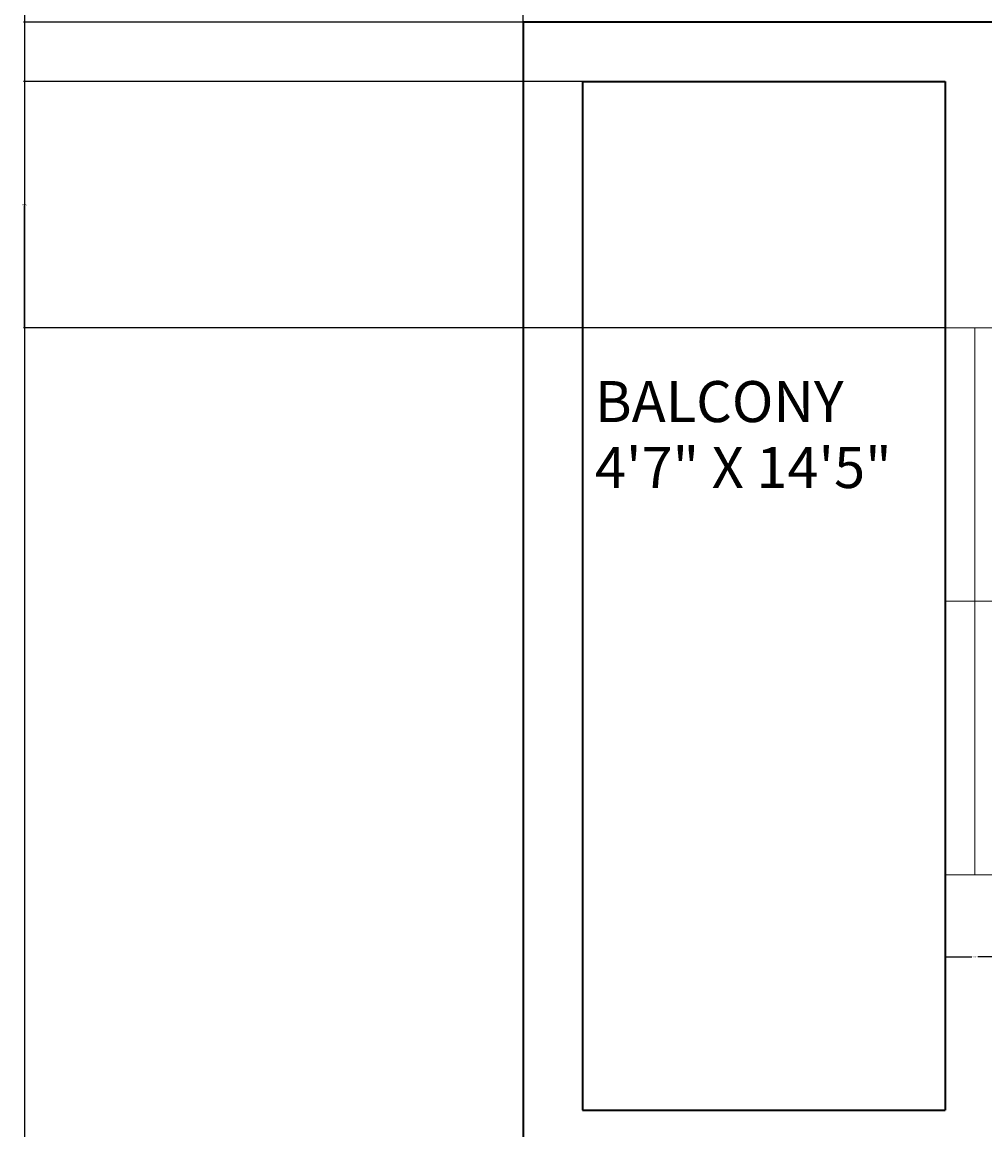
# Model space of a CAD drawing. Units: inches. Extents: x -61 to 1599, y -1316 to 257.
# Tile 112 of 204: x -61 to 85, y -10 to 158. Entities that reach past the tile are written whole.
import ezdxf

# ---------------------------------------------------------------- set-up
doc = ezdxf.new("R2010")
doc.units = ezdxf.units.IN
doc.header["$MEASUREMENT"] = 0
for name, color, linetype, lineweight in [('A-ANNO-DIMS', 2, 'Continuous', 18), ('A-AREA-IDEN', 1, 'Continuous', 18), ('WALLS', 4, 'Continuous', 35), ('WINDOWS', 220, 'Continuous', 18)]:
    doc.layers.add(name, color=color, linetype=linetype, lineweight=lineweight)
doc.styles.get("Standard").update_dxf_attribs({"font": 'arial.ttf'})
doc.dimstyles.get("Standard").update_dxf_attribs({"dimtxt": 0.18, "dimasz": 0.18, "dimexe": 0.18, "dimexo": 0.0625, "dimgap": 0.09, "dimtad": 0, "dimtih": 1, "dimtoh": 1, "dimdec": 0, "dimzin": 0, "dimdsep": 46, "dimlunit": 3, "dimtxsty": 'Standard', "dimcen": 0.09, "dimadec": 0, "dimazin": 0, "dimtfac": 1, "dimtdec": 0, "dimtofl": 0, "dimtmove": 0, "dimatfit": 3, "dimfxl": 1, "dimtolj": 1, "dimtzin": 0, "dimarcsym": 0})

# ---------------------------------------------------------------- blocks, each defined once
blk = doc.blocks.new('WIN-83IN')
for p, q in [((0, 82.94), (9, 82.94)), ((0, 0), (9, 0))]:
    blk.add_line(p, q)
for points in [[(9, 82.94), (4.5, 82.94), (4.5, 41.47), (9, 41.47)], [(4.5, 41.47), (0, 41.47), (0, 0), (4.5, 0)]]:
    blk.add_lwpolyline(points, close=True)
blk = doc.blocks.new('*D645')
at = {"layer": 'A-ANNO-DIMS', "color": 0, "lineweight": -2, "transparency": 16777216}
for p, q in [((78.7, 28.3), (78.7, 15.74)), ((87.7, 28.3), (87.7, 15.74)), ((78.88, 15.92), (82.74, 15.92)), ((87.52, 15.92), (83.66, 15.92))]:
    blk.add_line(p, q, dxfattribs=at)
at = {"layer": 'A-ANNO-DIMS', "color": 0, "transparency": 16777216}
for points in [[(78.88, 15.95), (78.88, 15.89), (78.7, 15.92)], [(87.52, 15.95), (87.52, 15.89), (87.7, 15.92)]]:
    blk.add_solid(points, dxfattribs=at)
at = {"layer": 'DEFPOINTS', "color": 0, "transparency": 16777216}
for p in [(78.7, 28.37), (87.7, 28.37), (87.7, 15.92)]:
    blk.add_point(p, dxfattribs=at)
at = {"layer": 'A-ANNO-DIMS', "color": 0, "transparency": 16777216, "insert": (83.2, 15.92), "char_height": 0.18, "attachment_point": 5}
blk.add_mtext('\\A1;9 TYP.', dxfattribs=at)
blk = doc.blocks.new('*D687')
at = {"layer": 'A-ANNO-DIMS', "color": 0, "lineweight": -2, "transparency": 16777216}
for p, q in [((289.42, 181.68), (-61.08, 181.68)), ((-60.9, 181.5), (-60.9, -528.95)), ((-60.9, -1239.76), (-60.9, -529.32)), ((319.64, -1239.94), (-61.08, -1239.94))]:
    blk.add_line(p, q, dxfattribs=at)
at = {"layer": 'A-ANNO-DIMS', "color": 0, "transparency": 16777216}
for points in [[(-60.93, 181.5), (-60.87, 181.5), (-60.9, 181.68)], [(-60.93, -1239.76), (-60.87, -1239.76), (-60.9, -1239.94)]]:
    blk.add_solid(points, dxfattribs=at)
at = {"layer": 'DEFPOINTS', "color": 0, "transparency": 16777216}
for p in [(289.48, 181.68), (-60.9, -1239.94), (319.7, -1239.94)]:
    blk.add_point(p, dxfattribs=at)
at = {"layer": 'A-ANNO-DIMS', "color": 0, "transparency": 16777216, "insert": (-60.9, -529.13), "char_height": 0.18, "attachment_point": 5}
blk.add_mtext('\\A1;1421.6', dxfattribs=at)
blk = doc.blocks.new('*D691')
at = {"layer": 'A-ANNO-DIMS', "color": 0, "lineweight": -2, "transparency": 16777216}
for p, q in [((14.64, 157.68), (-61.08, 157.68)), ((-60.9, 157.5), (-60.9, -141.64)), ((-60.9, -441.14), (-60.9, -142)), ((14.64, -441.32), (-61.08, -441.32))]:
    blk.add_line(p, q, dxfattribs=at)
at = {"layer": 'A-ANNO-DIMS', "color": 0, "transparency": 16777216}
for points in [[(-60.93, 157.5), (-60.87, 157.5), (-60.9, 157.68)], [(-60.93, -441.14), (-60.87, -441.14), (-60.9, -441.32)]]:
    blk.add_solid(points, dxfattribs=at)
at = {"layer": 'DEFPOINTS', "color": 0, "transparency": 16777216}
for p in [(-60.9, 157.68), (14.7, 157.68), (14.7, -441.32)]:
    blk.add_point(p, dxfattribs=at)
at = {"layer": 'A-ANNO-DIMS', "color": 0, "transparency": 16777216, "insert": (-60.9, -141.82), "char_height": 0.18, "attachment_point": 5}
blk.add_mtext('\\A1;599', dxfattribs=at)
blk = doc.blocks.new('*D700')
at = {"layer": 'A-ANNO-DIMS', "color": 0, "lineweight": -2, "transparency": 16777216}
for p, q in [((14.7, -616.88), (14.7, 257.46)), ((14.88, 257.28), (96.77, 257.28)), ((179.57, 257.28), (97.68, 257.28)), ((179.75, -616.88), (179.75, 257.46))]:
    blk.add_line(p, q, dxfattribs=at)
at = {"layer": 'A-ANNO-DIMS', "color": 0, "transparency": 16777216}
for points in [[(14.88, 257.31), (14.88, 257.25), (14.7, 257.28)], [(179.57, 257.31), (179.57, 257.25), (179.75, 257.28)]]:
    blk.add_solid(points, dxfattribs=at)
at = {"layer": 'DEFPOINTS', "color": 0, "transparency": 16777216}
for p in [(179.75, 257.28), (14.7, -616.94), (179.75, -616.94)]:
    blk.add_point(p, dxfattribs=at)
at = {"layer": 'A-ANNO-DIMS', "color": 0, "transparency": 16777216, "insert": (97.23, 257.28), "char_height": 0.18, "attachment_point": 5}
blk.add_mtext('\\A1;165.05', dxfattribs=at)
blk = doc.blocks.new('*D705')
at = {"layer": 'A-ANNO-DIMS', "color": 0, "lineweight": -2, "transparency": 16777216}
for p, q in [((78.64, 148.68), (-61.08, 148.68)), ((-60.9, 148.5), (-60.9, 130.17)), ((-60.9, 111.48), (-60.9, 129.81)), ((78.64, 111.3), (-61.08, 111.3))]:
    blk.add_line(p, q, dxfattribs=at)
at = {"layer": 'A-ANNO-DIMS', "color": 0, "transparency": 16777216}
for points in [[(-60.93, 148.5), (-60.87, 148.5), (-60.9, 148.68)], [(-60.93, 111.48), (-60.87, 111.48), (-60.9, 111.3)]]:
    blk.add_solid(points, dxfattribs=at)
at = {"layer": 'DEFPOINTS', "color": 0, "transparency": 16777216}
for p in [(-60.9, 148.68), (78.7, 148.68), (78.7, 111.3)]:
    blk.add_point(p, dxfattribs=at)
at = {"layer": 'A-ANNO-DIMS', "color": 0, "transparency": 16777216, "insert": (-60.9, 129.99), "char_height": 0.18, "attachment_point": 5}
blk.add_mtext('\\A1;37.376', dxfattribs=at)

msp = doc.modelspace()

# ---------------------------------------------------------------- linework, layer by layer
at = {"layer": 'WALLS'}
for p, q in [((14.7028, 157.6771), (14.7028, -441.3229)), ((544.7028, 157.6771), (14.7028, 157.6771)), ((23.7028, 148.6771), (23.7028, -7.3229)), ((23.7028, 148.6771), (78.7028, 148.6771)), ((78.7028, 148.6771), (78.7028, -7.3229)), ((23.7028, -7.3229), (78.7028, -7.3229))]:
    msp.add_line(p, q, dxfattribs=at)

# ---------------------------------------------------------------- block references
at = {"layer": 'WINDOWS'}
msp.add_blockref('WIN-83IN', (78.703, 28.365), dxfattribs=at)

# ---------------------------------------------------------------- texts
at = {"layer": 'A-AREA-IDEN'}
for s, height, p in [('BALCONY', 6.22364, (25.5954, 97.019)), ('4\'7" X 14\'5"', 6.223643, (25.5954, 87.0212))]:
    msp.add_text(s, height=height, dxfattribs=at).set_placement(p)

# ---------------------------------------------------------------- dimensions: what is measured, and where the dimension line sits
at = {"layer": 'A-ANNO-DIMS'}
dim = msp.add_linear_dim(base=(179.7521, 257.2771), p1=(14.7028, -616.9446), p2=(179.7521, -616.9446), dimstyle='Standard', override={"dimdec": 2, "dimlfac": 1, "dimrnd": 0, "dimzin": 0, "dimdsep": 46, "dimlunit": 2}, dxfattribs=at)
dim.commit()
dim.dimension.update_dxf_attribs({"geometry": '*D700', "text_midpoint": (97.2274, 257.2771)})
for base, p1, p2, override, picture, middle in [((-60.8972, -1239.9446), (289.4807, 181.6771), (319.7028, -1239.9446), {"dimdec": 1, "dimlfac": 1, "dimrnd": 0, "dimzin": 0, "dimdsep": 46, "dimlunit": 2}, '*D687', (-60.8972, -529.1337)), ((-60.8972, 157.6771), (14.7028, -441.3229), (14.7028, 157.6771), {"dimdec": 0, "dimlfac": 1, "dimrnd": 0, "dimzin": 0, "dimdsep": 46, "dimlunit": 2}, '*D691', (-60.8972, -141.8229)), ((-60.8972, 148.6771), (78.7028, 111.3013), (78.7028, 148.6771), {"dimdec": 3, "dimlfac": 1, "dimrnd": 0, "dimzin": 0, "dimdsep": 46, "dimlunit": 2}, '*D705', (-60.8972, 129.9892))]:
    dim = msp.add_linear_dim(base=base, p1=p1, p2=p2, angle=90, dimstyle='Standard', override=override, dxfattribs=at)
    dim.commit()
    dim.dimension.update_dxf_attribs({"geometry": picture, "text_midpoint": middle})
dim = msp.add_linear_dim(base=(87.7028, 15.9247), p1=(78.7028, 28.3651), p2=(87.7028, 28.3651), text='<> TYP.', dimstyle='Standard', override={"dimdec": 0, "dimlfac": 1, "dimrnd": 0, "dimzin": 0, "dimdsep": 46, "dimlunit": 2}, dxfattribs=at)
dim.commit()
dim.dimension.update_dxf_attribs({"geometry": '*D645', "text_midpoint": (83.2028, 15.9247)})

doc.saveas('drawing.dxf')
